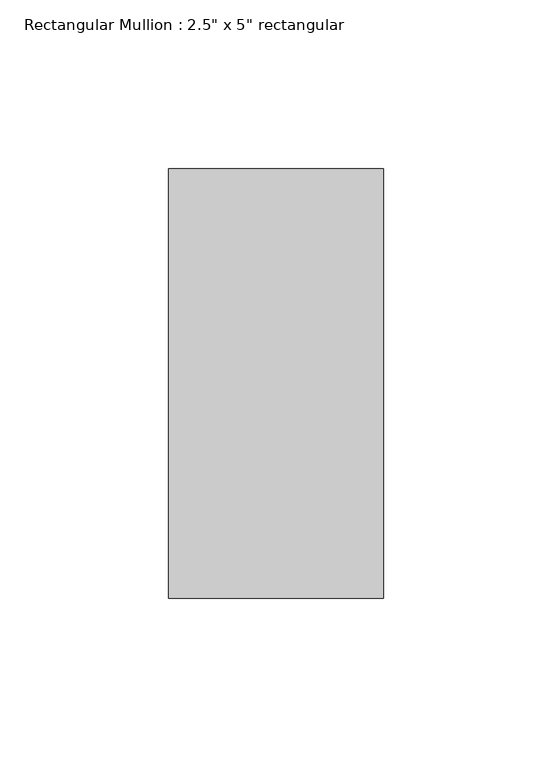
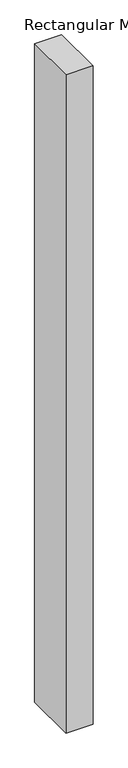
"""IFC4 building model written with IfcOpenShell, lengths in millimetres: member geometry."""

from ifc_helpers import new_model, si_unit, frame, origin, place, context, project, spatial, polyline, outline, extrude, source, transform, mapped, element, save


def member_517f38dd(model_context):
    return source(origin(), model_context, "Body", "SweptSolid", [
        extrude(outline(polyline([(31.75, 63.5), (31.75, -63.5), (-31.75, -63.5), (-31.75, 63.5), (31.75, 63.5)])), frame((0.0, 0.0, -1634.2331996), z_axis=(0.0, 0.0, 1.0), x_axis=(1.0, 0.0, 0.0)), (0.0, 0.0, 1.0), 1634.2331996),
    ])


if __name__ == "__main__":
    model = new_model("IFC4")
    model_context = context("Model", 3, world=origin())
    ifc_project = project(units=[si_unit("LENGTHUNIT", "METRE", prefix="MILLI")], contexts=[model_context])
    site = spatial("IfcSite", under=ifc_project)
    building = spatial("IfcBuilding", under=site)
    placement = place(None, origin())
    member_shape = member_517f38dd(model_context)
    element("IfcMember", 1, ObjectType="Rectangular Mullion : 2.5\" x 5\" rectangular", at=placement, inside=building, context=model_context, shape_type="MappedRepresentation", body=[
        mapped(member_shape, transform((0.0, 0.0, 0.0), x_axis=(1.0, 0.0, 0.0), y_axis=(0.0, 1.0, 0.0), z_axis=(0.0, 0.0, 1.0))),
    ])
    save(model, "model.ifc")

# Revit data of these elements
# Type "Rectangular Mullion : 2.5\" x 5\" rectangular"
#   built-in parameter 1007304 = 0.416667 (stored number, unit not read)
#   built-in parameter 1007301 = 0.104167 (stored number, unit not read)
#   built-in parameter 1007300 = 0.104167 (stored number, unit not read)
# Element 1 (IfcMember, "Rectangular Mullion : 2.5\" x 5\" rectangular")
#   Materials on its faces: "Aluminum"
# Materials
#   "Aluminum": class "Metal", colour RGB 247 247 247, transparency 0, Description = "Aluminum 6061", Cost = 0
